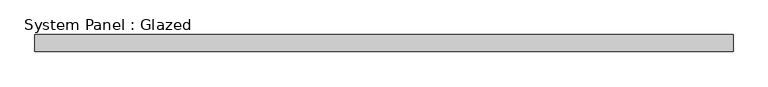
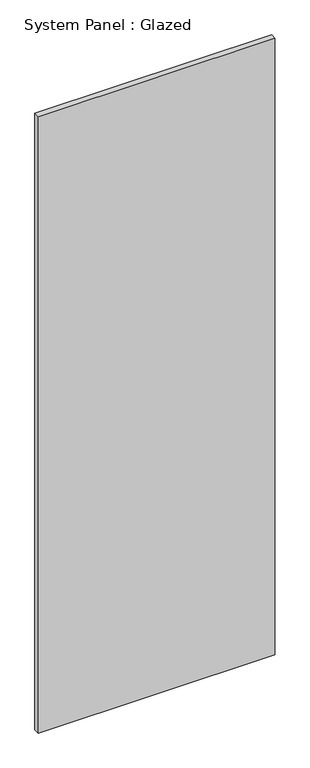
"""IFC4 building model written with IfcOpenShell, lengths in millimetres: plate geometry, System Panel : Glazed."""

from ifc_helpers import new_model, si_unit, origin, origin_with_axes, place, context, project, spatial, polyline, outline, extrude, source, transform, mapped, element, save


def system_panel_glazed_2efc79fa(model_context):
    return source(origin(), model_context, "Body", "SweptSolid", [
        extrude(outline(polyline([(523.875, 19.05), (-523.875, 19.05), (-523.875, 44.45), (523.875, 44.45), (523.875, 19.05)])), origin_with_axes(), (0.0, 0.0, 1.0), 2884.3632737),
    ])


if __name__ == "__main__":
    model = new_model("IFC4")
    model_context = context("Model", 3, world=origin())
    ifc_project = project(units=[si_unit("LENGTHUNIT", "METRE", prefix="MILLI")], contexts=[model_context])
    site = spatial("IfcSite", under=ifc_project)
    building = spatial("IfcBuilding", under=site)
    placement = place(None, origin())
    system_panel_glazed_shape = system_panel_glazed_2efc79fa(model_context)
    element("IfcPlate", 1, ObjectType="System Panel : Glazed", at=placement, inside=building, context=model_context, shape_type="MappedRepresentation", body=[
        mapped(system_panel_glazed_shape, transform((0.0, 0.0, 0.0), x_axis=(1.0, 0.0, 0.0), y_axis=(0.0, 1.0, 0.0), z_axis=(0.0, 0.0, 1.0))),
    ])
    save(model, "model.ifc")

# Revit data of these elements
# Type "System Panel : Glazed"
#   Construction Type Id = "GSP4R"
#   Analytic Construction = "1/8 in Pilkington single glazing"
#   Visual Light Transmittance = 0.9
#   Solar Heat Gain Coefficient = 0.86
#   Heat Transfer Coefficient (U) = 1.18115 BTU/(h·ft²·°F)
#   Define Thermal Properties by = 1
# Element 1 (IfcPlate, "System Panel : Glazed")
#   Materials on its faces: "Glass"
# Materials
#   "Glass": class "Glass", colour RGB 0 128 192, transparency 0.75, Description = "Soda Lime Glass", Cost = 0
